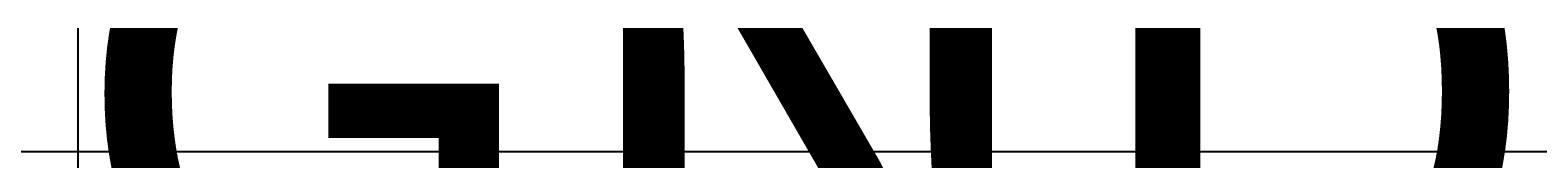
# Model space of a CAD drawing. Units: inches. Extents: x 35362 to 73946, y 43607 to 67532.
# Tile 96 of 134: x 50119 to 50761, y 48917 to 48969. Entities that reach past the tile are written whole.
import ezdxf

# ---------------------------------------------------------------- set-up
doc = ezdxf.new("R2010")
doc.units = ezdxf.units.IN
doc.header["$MEASUREMENT"] = 0
doc.layers.add('A-ANNO-DIMS', color=2, linetype='Continuous', lineweight=18)
doc.layers.add('E-ANNO-TEXT', color=5, linetype='Continuous', lineweight=18)
doc.styles.get("Standard").update_dxf_attribs({"font": 'arial.ttf'})
doc.dimstyles.get("Standard").update_dxf_attribs({"dimtxt": 0.18, "dimasz": 0.18, "dimexe": 0.18, "dimexo": 0.0625, "dimgap": 0.09, "dimtad": 0, "dimtih": 1, "dimtoh": 1, "dimdec": 4, "dimzin": 0, "dimdsep": 46, "dimtxsty": 'Standard', "dimcen": 0.09, "dimadec": 0, "dimazin": 0, "dimtfac": 1, "dimtdec": 4, "dimtofl": 0, "dimtmove": 0, "dimatfit": 3, "dimfxl": 1, "dimtolj": 1, "dimtzin": 0, "dimarcsym": 0})

# ---------------------------------------------------------------- blocks, each defined once
blk = doc.blocks.new('*D11')
at = {"layer": 'A-ANNO-DIMS', "color": 0, "lineweight": -2, "transparency": 16777216}
for p, q in [((47978.66, 56028.77), (47978.66, 43606.68)), ((53109.76, 56028.77), (53109.76, 43606.68)), ((47978.84, 43606.86), (50543.87, 43606.86)), ((53109.58, 43606.86), (50544.55, 43606.86))]:
    blk.add_line(p, q, dxfattribs=at)
at = {"layer": 'A-ANNO-DIMS', "color": 0, "transparency": 16777216}
for points in [[(47978.84, 43606.89), (47978.84, 43606.83), (47978.66, 43606.86)], [(53109.58, 43606.89), (53109.58, 43606.83), (53109.76, 43606.86)]]:
    blk.add_solid(points, dxfattribs=at)
at = {"layer": 'Defpoints', "color": 0, "transparency": 16777216}
for p in [(47978.66, 56028.84), (53109.76, 56028.84), (53109.76, 43606.86)]:
    blk.add_point(p, dxfattribs=at)
at = {"layer": 'A-ANNO-DIMS', "color": 0, "transparency": 16777216, "insert": (50544.21, 43606.86), "char_height": 0.18, "attachment_point": 5}
blk.add_mtext('\\A1;5131', dxfattribs=at)
blk = doc.blocks.new('*D13')
at = {"layer": 'A-ANNO-DIMS', "color": 0, "lineweight": -2, "transparency": 16777216}
for p, q in [((48373.49, 51694.02), (48373.49, 43606.68)), ((51029.04, 51694.02), (51029.04, 43606.68)), ((48373.67, 43606.86), (49700.8, 43606.86)), ((51028.86, 43606.86), (49701.73, 43606.86))]:
    blk.add_line(p, q, dxfattribs=at)
at = {"layer": 'A-ANNO-DIMS', "color": 0, "transparency": 16777216}
for points in [[(48373.67, 43606.89), (48373.67, 43606.83), (48373.49, 43606.86)], [(51028.86, 43606.89), (51028.86, 43606.83), (51029.04, 43606.86)]]:
    blk.add_solid(points, dxfattribs=at)
at = {"layer": 'Defpoints', "color": 0, "transparency": 16777216}
for p in [(48373.49, 51694.09), (51029.04, 51694.09), (51029.04, 43606.86)]:
    blk.add_point(p, dxfattribs=at)
at = {"layer": 'A-ANNO-DIMS', "color": 0, "transparency": 16777216, "insert": (49701.27, 43606.86), "char_height": 0.18, "attachment_point": 5}
blk.add_mtext('\\A1;2655.6', dxfattribs=at)
blk = doc.blocks.new('*D17')
at = {"layer": 'A-ANNO-DIMS', "color": 0, "lineweight": -2, "transparency": 16777216}
for p, q in [((49923.31, 61293.22), (49923.31, 43606.68)), ((51913.93, 61293.22), (51913.93, 43606.68)), ((49923.49, 43606.86), (50918.16, 43606.86)), ((51913.75, 43606.86), (50919.07, 43606.86))]:
    blk.add_line(p, q, dxfattribs=at)
at = {"layer": 'A-ANNO-DIMS', "color": 0, "transparency": 16777216}
for points in [[(49923.49, 43606.89), (49923.49, 43606.83), (49923.31, 43606.86)], [(51913.75, 43606.89), (51913.75, 43606.83), (51913.93, 43606.86)]]:
    blk.add_solid(points, dxfattribs=at)
at = {"layer": 'Defpoints', "color": 0, "transparency": 16777216}
for p in [(49923.31, 61293.29), (51913.93, 61293.29), (51913.93, 43606.86)]:
    blk.add_point(p, dxfattribs=at)
at = {"layer": 'A-ANNO-DIMS', "color": 0, "transparency": 16777216, "insert": (50918.62, 43606.86), "char_height": 0.18, "attachment_point": 5}
blk.add_mtext('\\A1;1990.6', dxfattribs=at)
blk = doc.blocks.new('*D67')
at = {"layer": 'A-ANNO-DIMS', "color": 0, "lineweight": -2, "transparency": 16777216}
for p, q in [((56873.54, 53351.53), (35361.77, 53351.53)), ((35361.95, 53351.35), (35361.95, 49400.89)), ((35361.95, 45450.07), (35361.95, 49400.53)), ((53793.58, 45449.89), (35361.77, 45449.89))]:
    blk.add_line(p, q, dxfattribs=at)
at = {"layer": 'A-ANNO-DIMS', "color": 0, "transparency": 16777216}
for points in [[(35361.92, 53351.35), (35361.98, 53351.35), (35361.95, 53351.53)], [(35361.92, 45450.07), (35361.98, 45450.07), (35361.95, 45449.89)]]:
    blk.add_solid(points, dxfattribs=at)
at = {"layer": 'Defpoints', "color": 0, "transparency": 16777216}
for p in [(35361.95, 53351.53), (56873.6, 53351.53), (53793.64, 45449.89)]:
    blk.add_point(p, dxfattribs=at)
at = {"layer": 'A-ANNO-DIMS', "color": 0, "transparency": 16777216, "insert": (35361.95, 49400.71), "char_height": 0.18, "attachment_point": 5}
blk.add_mtext('\\A1;7901.6', dxfattribs=at)
blk = doc.blocks.new('*D86')
at = {"layer": 'A-ANNO-DIMS', "color": 0, "lineweight": -2, "transparency": 16777216}
for p, q in [((51285.53, 49320.08), (35361.77, 49320.08)), ((35361.95, 49319.9), (35361.95, 49120.26)), ((35361.95, 48920.26), (35361.95, 49119.9)), ((51285.53, 48920.08), (35361.77, 48920.08))]:
    blk.add_line(p, q, dxfattribs=at)
at = {"layer": 'A-ANNO-DIMS', "color": 0, "transparency": 16777216}
for points in [[(35361.92, 49319.9), (35361.98, 49319.9), (35361.95, 49320.08)], [(35361.92, 48920.26), (35361.98, 48920.26), (35361.95, 48920.08)]]:
    blk.add_solid(points, dxfattribs=at)
at = {"layer": 'Defpoints', "color": 0, "transparency": 16777216}
for p in [(35361.95, 49320.08), (51285.59, 49320.08), (51285.59, 48920.08)]:
    blk.add_point(p, dxfattribs=at)
at = {"layer": 'A-ANNO-DIMS', "color": 0, "transparency": 16777216, "insert": (35361.95, 49120.08), "char_height": 0.18, "attachment_point": 5}
blk.add_mtext('\\A1;400.0', dxfattribs=at)
blk = doc.blocks.new('*D107')
at = {"layer": 'A-ANNO-DIMS', "color": 0, "lineweight": -2, "transparency": 16777216}
for p, q in [((50139.56, 59850.01), (50139.56, 43606.68)), ((51320.81, 59850.01), (51320.81, 43606.68)), ((50139.74, 43606.86), (50729.73, 43606.86)), ((51320.63, 43606.86), (50730.64, 43606.86))]:
    blk.add_line(p, q, dxfattribs=at)
at = {"layer": 'A-ANNO-DIMS', "color": 0, "transparency": 16777216}
for points in [[(50139.74, 43606.89), (50139.74, 43606.83), (50139.56, 43606.86)], [(51320.63, 43606.89), (51320.63, 43606.83), (51320.81, 43606.86)]]:
    blk.add_solid(points, dxfattribs=at)
at = {"layer": 'Defpoints', "color": 0, "transparency": 16777216}
for p in [(50139.56, 59850.08), (51320.81, 59850.08), (51320.81, 43606.86)]:
    blk.add_point(p, dxfattribs=at)
at = {"layer": 'A-ANNO-DIMS', "color": 0, "transparency": 16777216, "insert": (50730.19, 43606.86), "char_height": 0.18, "attachment_point": 5}
blk.add_mtext('\\A1;1181.3', dxfattribs=at)

msp = doc.modelspace()

# ---------------------------------------------------------------- texts
at = {"layer": 'E-ANNO-TEXT'}
msp.add_text('GND', height=220.866, dxfattribs=at).set_placement((50133.331, 48834.598))

# ---------------------------------------------------------------- dimensions: what is measured, and where the dimension line sits
at = {"layer": 'A-ANNO-DIMS'}
for base, p1, p2, override, picture, middle in [((51913.931, 43606.859), (49923.307, 61293.286), (51913.931, 61293.286), {"dimdec": 1, "dimlfac": 1, "dimrnd": 0, "dimzin": 0, "dimdsep": 46, "dimlunit": 2}, '*D17', (50918.619, 43606.859)), ((51320.8133, 43606.859), (50139.5627, 59850.0769), (51320.8133, 59850.0769), {"dimdec": 1, "dimlfac": 1, "dimrnd": 0, "dimzin": 0, "dimdsep": 46, "dimlunit": 2}, '*D107', (50730.188, 43606.859)), ((53109.76, 43606.859), (47978.665, 56028.836), (53109.76, 56028.836), {"dimdec": 0, "dimlfac": 1, "dimrnd": 0, "dimzin": 0, "dimdsep": 46, "dimlunit": 2}, '*D11', (50544.212, 43606.859)), ((51029.043, 43606.859), (48373.492, 51694.087), (51029.043, 51694.087), {"dimdec": 1, "dimlfac": 1, "dimrnd": 0, "dimzin": 0, "dimdsep": 46, "dimlunit": 2}, '*D13', (49701.267, 43606.859))]:
    dim = msp.add_linear_dim(base=base, p1=p1, p2=p2, dimstyle='Standard', override=override, dxfattribs=at)
    dim.commit()
    dim.dimension.update_dxf_attribs({"geometry": picture, "text_midpoint": middle})
for base, p1, p2, picture, middle in [((35361.949, 53351.529), (53793.638, 45449.894), (56873.602, 53351.529), '*D67', (35361.949, 49400.712)), ((35361.949, 49320.079), (51285.595, 48920.079), (51285.595, 49320.079), '*D86', (35361.949, 49120.079))]:
    dim = msp.add_linear_dim(base=base, p1=p1, p2=p2, angle=90, dimstyle='Standard', override={"dimdec": 1, "dimlfac": 1, "dimrnd": 0, "dimzin": 0, "dimdsep": 46, "dimlunit": 2}, dxfattribs=at)
    dim.commit()
    dim.dimension.update_dxf_attribs({"geometry": picture, "text_midpoint": middle})

doc.saveas('drawing.dxf')
